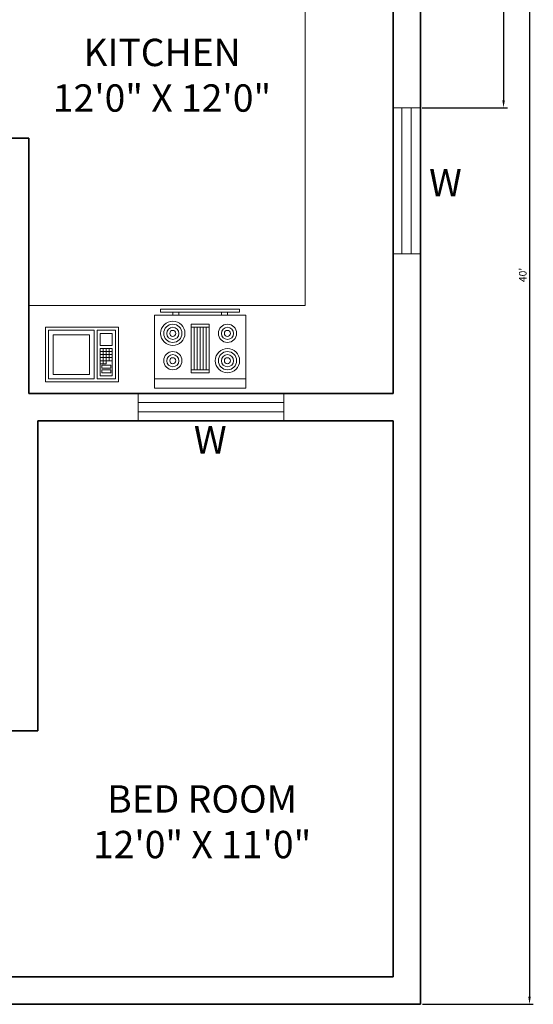
# Model space of a CAD drawing. Units: inches. Extents: x 1025 to 3479, y 1594 to 2212.
# Tile 5 of 9: x 2572 to 2741, y 1623 to 1947. Entities that reach past the tile are written whole.
import ezdxf

# ---------------------------------------------------------------- set-up
doc = ezdxf.new("R2010")
doc.units = ezdxf.units.IN
for name, color, linetype, lineweight in [('A-ANNO-DIMS', 1, 'Continuous', 18), ('A-ANNO-TEXT', 7, 'Continuous', 18), ('A-AREA-IDEN', 4, 'Continuous', 18), ('A-EQPM', 9, 'Continuous', 18), ('A-FLOR-CSWK', 8, 'Continuous', 18), ('A-GLAZ', 3, 'Continuous', 18), ('A-WALL', 7, 'Continuous', 35)]:
    doc.layers.add(name, color=color, linetype=linetype, lineweight=lineweight)
doc.styles.get("Standard").update_dxf_attribs({"font": 'arial.ttf'})
doc.dimstyles.new('ISO-25', dxfattribs={"dimtxt": 2.5, "dimasz": 2.5, "dimexe": 1.25, "dimexo": 0.625, "dimtad": 1, "dimdec": 0, "dimlunit": 3, "dimtxsty": 'Standard', "dimcen": 2.5, "dimadec": 0, "dimazin": 0, "dimtfac": 1, "dimtdec": 0, "dimtmove": 0, "dimatfit": 3, "dimfxl": 1, "dimarcsym": 0})

# ---------------------------------------------------------------- blocks, each defined once
blk = doc.blocks.new('*D5')
at = {"layer": 'A-ANNO-DIMS', "color": 0, "lineweight": -2, "transparency": 16777216}
for p, q in [((2704.45, 2102.86), (2740.97, 2102.86)), ((2739.72, 2100.36), (2739.72, 1625.36)), ((2704.45, 1622.86), (2740.97, 1622.86))]:
    blk.add_line(p, q, dxfattribs=at)
at = {"layer": 'A-ANNO-DIMS', "color": 0, "transparency": 16777216}
for points in [[(2739.31, 2100.36), (2740.14, 2100.36), (2739.72, 2102.86)], [(2739.31, 1625.36), (2740.14, 1625.36), (2739.72, 1622.86)]]:
    blk.add_solid(points, dxfattribs=at)
at = {"layer": 'Defpoints', "color": 0, "transparency": 16777216}
for p in [(2703.82, 2102.86), (2703.82, 1622.86), (2739.72, 1622.86)]:
    blk.add_point(p, dxfattribs=at)
at = {"layer": 'A-ANNO-DIMS', "color": 0, "transparency": 16777216, "insert": (2737.82, 1862.86), "char_height": 2.5, "attachment_point": 5, "rotation": 90}
blk.add_mtext("40'", dxfattribs=at)
blk = doc.blocks.new('Range-Oven - 30 in top')
for p, q in [((0, -3), (30, -3)), ((12, -6), (18, -6)), ((13, -20), (13, -6)), ((14, -6), (14, -20)), ((15, -20), (15, -6)), ((16, -6), (16, -20)), ((17, -20), (17, -6)), ((18, -20), (12, -20)), ((6, -24), (6, -25)), ((8, -25), (8, -24)), ((22, -25), (22, -24)), ((24, -24), (24, -25))]:
    blk.add_line(p, q)
for points in [[(0, -24), (0, 0), (30, 0), (30, -24)], [(12, -21), (12, -5), (18, -5), (18, -21)], [(2, -26), (2, -25), (28, -25), (28, -26)]]:
    blk.add_lwpolyline(points, close=True)
for centre, radius in [((6, -9), 4), ((6, -9), 3), ((24, -9), 3), ((6, -9), 2), ((6, -9), 1), ((24, -9), 2), ((24, -9), 1), ((6, -18), 3), ((6, -18), 2), ((24, -18), 4), ((24, -18), 3), ((24, -18), 2), ((6, -18), 1), ((24, -18), 1)]:
    blk.add_circle(centre, radius)
blk = doc.blocks.new('Microwave')
for p, q in [((18, 10), (22, 10)), ((19, 7), (19, 11)), ((20, 11), (20, 7)), ((21, 7), (21, 11)), ((22, 9), (18, 9)), ((18, 8), (22, 8)), ((22, 7), (18, 7)), ((19, 6), (19, 7)), ((20, 7), (20, 6)), ((20, 6), (18, 6))]:
    blk.add_line(p, q)
for points in [[(0, 0), (0, 18), (24, 18), (24, 0)], [(1, 1), (1, 17), (16, 17), (16, 1)], [(17, 1), (17, 17), (23, 17), (23, 1)], [(2.5, 2.5), (2.5, 15.5), (14.5, 15.5), (14.5, 2.5)], [(18, 12), (18, 16), (22, 16), (22, 12)], [(18, 2), (18, 11), (22, 11), (22, 2)], [(18.5, 4.5), (18.5, 5.5), (21.5, 5.5), (21.5, 4.5)], [(18.5, 3), (18.5, 4), (21.5, 4), (21.5, 3)]]:
    blk.add_lwpolyline(points, close=True)
blk = doc.blocks.new('WIN-48IN')
for p, q in [((0, 48), (0, 0)), ((9, 48), (0, 48)), ((3, 48), (3, 0)), ((6, 0), (6, 48)), ((9, 0), (9, 48)), ((0, 0), (9, 0))]:
    blk.add_line(p, q)
blk = doc.blocks.new('*D75')
at = {"layer": 'A-ANNO-DIMS', "color": 0, "lineweight": -2, "transparency": 16777216}
for p, q in [((2704.38, 2007.25), (2732.42, 2007.25)), ((2731.17, 2004.75), (2731.17, 1920.36)), ((2704.35, 1917.86), (2732.42, 1917.86))]:
    blk.add_line(p, q, dxfattribs=at)
at = {"layer": 'A-ANNO-DIMS', "color": 0, "transparency": 16777216}
for points in [[(2730.76, 2004.75), (2731.59, 2004.75), (2731.17, 2007.25)], [(2730.76, 1920.36), (2731.59, 1920.36), (2731.17, 1917.86)]]:
    blk.add_solid(points, dxfattribs=at)
at = {"layer": 'Defpoints', "color": 0, "transparency": 16777216}
for p in [(2703.75, 2007.25), (2703.72, 1917.86), (2731.17, 1917.86)]:
    blk.add_point(p, dxfattribs=at)
at = {"layer": 'A-ANNO-DIMS', "color": 0, "transparency": 16777216, "insert": (2729.26, 1962.56), "char_height": 2.5, "attachment_point": 5, "rotation": 90}
blk.add_mtext('7\'-5 1/2"', dxfattribs=at)

msp = doc.modelspace()

# ---------------------------------------------------------------- linework, layer by layer
at = {"layer": 'A-FLOR-CSWK'}
for p in [(2665.82, 1967.86), (2574.82, 1852.86)]:
    msp.add_line(p, (2665.82, 1852.86), dxfattribs=at)
at = {"layer": 'A-WALL'}
for p, q in [((2703.82, 2102.86), (2703.82, 1622.86)), ((2694.82, 1967.86), (2694.82, 1823.86)), ((2574.82, 1907.86), (2568.82, 1907.86)), ((2574.82, 1895.86), (2574.82, 1907.86)), ((2574.82, 1823.86), (2574.82, 1895.86)), ((2574.82, 1823.86), (2694.82, 1823.86)), ((2577.82, 1814.86), (2694.82, 1814.86)), ((2577.82, 1712.86), (2577.82, 1814.86)), ((2694.82, 1814.86), (2694.82, 1631.86)), ((2568.82, 1712.86), (2577.82, 1712.86)), ((2694.82, 1631.86), (2352.82, 1631.86)), ((2703.82, 1622.86), (2343.82, 1622.86))]:
    msp.add_line(p, q, dxfattribs=at)

# ---------------------------------------------------------------- block references
at = {"layer": 'A-EQPM', "rotation": 180}
msp.add_blockref('Range-Oven - 30 in top', (2646.25, 1825.64), dxfattribs=at)
at = {"layer": 'A-EQPM'}
msp.add_blockref('Microwave', (2580.33, 1827.65), dxfattribs=at)
at = {"layer": 'A-GLAZ'}
msp.add_blockref('WIN-48IN', (2694.72, 1869.86), dxfattribs=at)
at = {"layer": 'A-GLAZ', "rotation": 270.0000000000003}
msp.add_blockref('WIN-48IN', (2610.82, 1823.86), dxfattribs=at)

# ---------------------------------------------------------------- texts
at = {"layer": 'A-ANNO-TEXT', "char_height": 9, "attachment_point": 1}
for insert in [(2704.1, 1897.76), (2626.64, 1813.11)]:
    msp.add_mtext_dynamic_manual_height_columns('\\pxqc;W', width=15.8719, gutter_width=12.5, heights=[0], dxfattribs=dict(at, insert=insert))
at = {"layer": 'A-AREA-IDEN', "char_height": 9, "attachment_point": 1}
for s, insert in [('\\pxqc;KITCHEN \\P12\'0" X 12\'0"', (2572.08, 1940.59)), ('\\pxqc;BED ROOM \\P12\'0" X 11\'0"', (2585.29, 1694.93))]:
    msp.add_mtext_dynamic_manual_height_columns(s, width=93.2353, gutter_width=12.5, heights=[0], dxfattribs=dict(at, insert=insert))

# ---------------------------------------------------------------- dimensions: what is measured, and where the dimension line sits
at = {"layer": 'A-ANNO-DIMS'}
for base, p1, p2, override, picture, middle in [((2739.72, 1622.86), (2703.82, 2102.86), (2703.82, 1622.86), {"dimclrd": 0, "dimclre": 0, "dimclrt": 0}, '*D5', (2737.82, 1862.86)), ((2731.17, 1917.86), (2703.75, 2007.25), (2703.72, 1917.86), {"dimdec": 1, "dimlfac": 1, "dimrnd": 0, "dimzin": 1, "dimdsep": 46, "dimlunit": 4, "dimfrac": 2}, '*D75', (2729.26, 1962.56))]:
    dim = msp.add_linear_dim(base=base, p1=p1, p2=p2, angle=90, dimstyle='ISO-25', override=override, dxfattribs=at)
    dim.commit()
    dim.dimension.update_dxf_attribs({"geometry": picture, "text_midpoint": middle})

doc.saveas('drawing.dxf')
